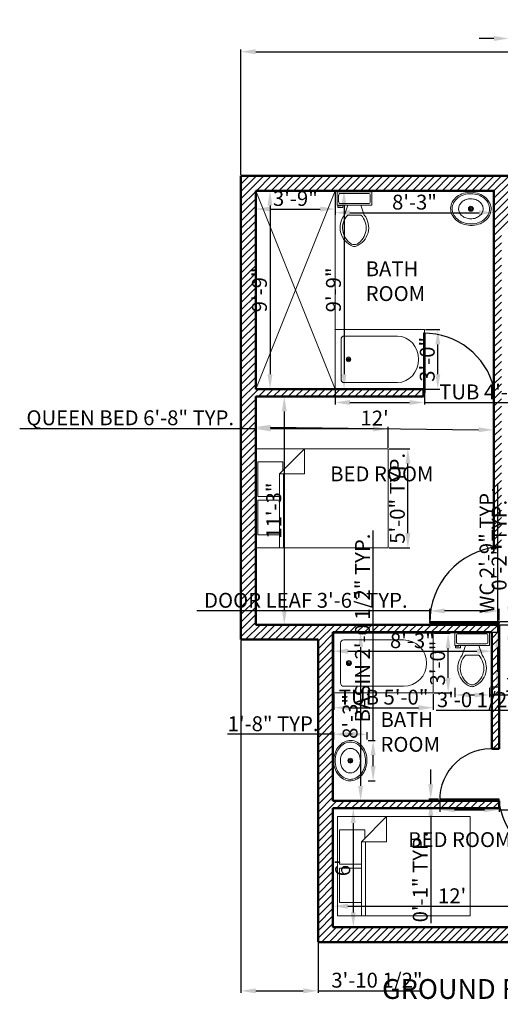
# Model space of a CAD drawing. Units: inches. Extents: x 5928 to 6612, y 5674 to 6320.
# Tile 1 of 5: x 5928 to 6219, y 5674 to 6269. Entities that reach past the tile are written whole.
import ezdxf

# ---------------------------------------------------------------- set-up
doc = ezdxf.new("R2010")
doc.units = ezdxf.units.IN
for name, color, linetype, lineweight in [('A-ANNO-DIMS', 2, 'Continuous', 18), ('A-ANNO-TEXT', 7, 'Continuous', 25), ('A-AREA-IDEN', 7, 'Continuous', 25), ('A-DOOR', 3, 'Continuous', 25), ('A-FLOR-FIXT', 9, 'Continuous', 18), ('A-FLOR-OPEN', 8, 'Continuous', 18), ('A-FURN', 8, 'Continuous', 18), ('A-WALL', 7, 'Continuous', 50), ('A-WALL-PATT', 252, 'Continuous', 13)]:
    doc.layers.add(name, color=color, linetype=linetype, lineweight=lineweight)
doc.styles.get("Standard").update_dxf_attribs({"font": 'arial.ttf'})
doc.dimstyles.new('ISO-25', dxfattribs={"dimtxt": 9, "dimasz": 9, "dimexe": 1.25, "dimexo": 0.625, "dimtad": 1, "dimdec": 1, "dimrnd": 9, "dimlunit": 3, "dimtxsty": 'Standard', "dimcen": 2.5, "dimadec": 0, "dimazin": 0, "dimtfac": 1, "dimtdec": 1, "dimtmove": 0, "dimatfit": 3, "dimfxl": 1, "dimarcsym": 0})

# ---------------------------------------------------------------- blocks, each defined once
blk = doc.blocks.new('Bed - Queen')
for p, q in [((0, -80.00003), (0, 0)), ((0, 0), (59.99999, 0)), ((59.99999, 0), (59.99999, -80.00003)), ((7.99999, -1.2), (28.79998, -1.2)), ((7.99999, -14.4), (7.99999, -1.2)), ((28.79998, -1.2), (28.79998, -14.4)), ((31.19999, -1.2), (51.99999, -1.2)), ((31.19999, -14.4), (31.19999, -1.2)), ((51.99999, -1.2), (51.99999, -16.4)), ((0, -14.4), (44.8, -14.4)), ((44.8, -16.8), (0, -16.8)), ((59.99999, -29.6), (44.8, -14.4)), ((44.8, -14.4), (44.8, -29.6)), ((51.99999, -16.4), (46.79936, -16.4)), ((44.8, -29.6), (59.99999, -29.6)), ((59.99999, -80.00003), (0, -80.00003))]:
    blk.add_line(p, q)
blk = doc.blocks.new('Toilet - top')
for p, q in [((9.5, -6), (9.5, -2)), ((-10, -8.5), (-8, -8.5)), ((-10, -9.5), (-10, -8.5)), ((-7, -9.5), (-10, -9.5)), ((-8, -8.5), (-8, -8)), ((-7, -8), (-7, -9.5)), ((-4, -8), (-6, -14)), ((4, -8), (6, -14)), ((4, -14), (-4, -14))]:
    blk.add_line(p, q)
blk.add_lwpolyline([(10.5, -8), (10.5, 0), (-10.5, 0), (-10.5, -8)], close=True)
for points in [[(-9.5, -2), (-9.5, -6)], [(8.5, -1), (-8.5, -1)], [(-8.5, -7), (8.5, -7)]]:
    blk.add_lwpolyline(points)
for centre, radius, start, end in [((-8.62, -1.88), 0.884, 81.8699, 188.1301), ((8.62, -1.88), 0.884, 351.8699, 98.1301), ((-8.62, -6.12), 0.884, 171.8699, 278.1301), ((8.62, -6.12), 0.884, 261.8699, 8.1301), ((3.52, -21.58), 12.17, 141.46911, 247.97143), ((4.2, -21.82), 11.33, 136.36773, 238.94682), ((-3.52, -21.58), 12.17, 292.02843, 38.53071), ((-4.2, -21.82), 11.33, 301.05301, 43.63209), ((0, -27.88), 4, 245.73182, 294.26817), ((0, -29), 4, 254.86053, 285.13947)]:
    blk.add_arc(centre, radius, start, end)
blk = doc.blocks.new('Bath Tub - 26 x 60 in.')
for p, q in [((9, -17), (9, -19)), ((8, -18), (10, -18))]:
    blk.add_line(p, q)
blk.add_lwpolyline([(0, -36), (0, 0), (60, 0), (60, -36)], close=True)
for points in [[(6, -4), (42, -4)], [(4, -30), (4, -6)], [(42, -32), (6, -32)]]:
    blk.add_lwpolyline(points)
for radius in [1.5, 1]:
    blk.add_circle((9, -18), radius)
for centre, radius, start, end in [((5.75, -5.75), 1.77, 81.8699, 188.1301), ((42, -18), 14, 270, 90), ((5.75, -30.25), 1.77, 171.8699, 278.1301)]:
    blk.add_arc(centre, radius, start, end)
blk = doc.blocks.new('Sink - Oval top')
for p, q in [((-1, 0), (1, 0)), ((0, 1), (0, -1))]:
    blk.add_line(p, q)
for points in [[(-12.23, 0.39, 0.117634), (-11.46, -3.36, 0.104469), (-8.88, -6.8, 0.090016), (-5.08, -9.07, 0.08192), (-0.32, -10.02, 0.08192), (4.49, -9.38, 0.090016), (8.42, -7.36, 0.104469), (11.22, -4.09, 0.117634), (12.23, -0.39, 0.117634), (11.46, 3.36, 0.104469), (8.88, 6.8, 0.090016), (5.08, 9.07, 0.08192), (0.32, 10.02, 0.08192), (-4.49, 9.38, 0.090016), (-8.42, 7.36, 0.104469), (-11.22, 4.09, 0.117634)], [(-11.29, 0.16, 0.118622), (-10.52, -3.25, 0.104678), (-8.07, -6.36, 0.089562), (-4.54, -8.37, 0.081185), (-0.13, -9.15, 0.081185), (4.3, -8.49, 0.089562), (7.89, -6.58, 0.104678), (10.42, -3.55, 0.118622), (11.29, -0.16, 0.118622), (10.52, 3.25, 0.104678), (8.07, 6.36, 0.089562), (4.54, 8.37, 0.081185), (0.13, 9.15, 0.081185), (-4.3, 8.49, 0.089562), (-7.89, 6.58, 0.104678), (-10.42, 3.55, 0.118622)], [(-7.42, 0.08, 0.118283), (-6.91, -2.17, 0.104607), (-5.29, -4.21, 0.089718), (-2.97, -5.53, 0.081436), (-0.07, -6.04, 0.081436), (2.84, -5.59, 0.089718), (5.2, -4.33, 0.104607), (6.86, -2.32, 0.118283), (7.42, -0.08, 0.118283), (6.91, 2.17, 0.104607), (5.29, 4.21, 0.089718), (2.97, 5.53, 0.081436), (0.07, 6.04, 0.081436), (-2.84, 5.59, 0.089718), (-5.2, 4.33, 0.104607), (-6.86, 2.32, 0.118283)]]:
    blk.add_lwpolyline(points, format="xyb", close=True)
for radius in [1.5, 1]:
    blk.add_circle((0, 0), radius)
blk = doc.blocks.new('*D11')
at = {"layer": 'A-ANNO-DIMS', "color": 0, "lineweight": -2, "transparency": 16777216}
for p, q in [((6071.65, 6165.76), (6080.95, 6165.76)), ((6079.7, 6156.76), (6079.7, 6054.76)), ((6071.65, 6045.76), (6080.95, 6045.76))]:
    blk.add_line(p, q, dxfattribs=at)
at = {"layer": 'A-ANNO-DIMS', "color": 0, "transparency": 16777216}
for points in [[(6078.2, 6156.76), (6081.2, 6156.76), (6079.7, 6165.76)], [(6078.2, 6054.76), (6081.2, 6054.76), (6079.7, 6045.76)]]:
    blk.add_solid(points, dxfattribs=at)
at = {"layer": 'Defpoints', "color": 0, "transparency": 16777216}
for p in [(6071.03, 6165.76), (6071.03, 6045.76), (6079.7, 6045.76)]:
    blk.add_point(p, dxfattribs=at)
at = {"layer": 'A-ANNO-DIMS', "color": 0, "transparency": 16777216, "insert": (6074.47, 6105.76), "char_height": 9, "attachment_point": 5, "rotation": 90}
blk.add_mtext('9\'-9"', dxfattribs=at)
blk = doc.blocks.new('*D12')
at = {"layer": 'A-ANNO-DIMS', "color": 0, "lineweight": -2, "transparency": 16777216}
for p, q in [((6071.03, 6165.14), (6071.03, 6153.42)), ((6119.03, 6165.14), (6119.03, 6153.42)), ((6080.03, 6154.67), (6110.03, 6154.67))]:
    blk.add_line(p, q, dxfattribs=at)
at = {"layer": 'A-ANNO-DIMS', "color": 0, "transparency": 16777216}
for points in [[(6080.03, 6156.17), (6080.03, 6153.17), (6071.03, 6154.67)], [(6110.03, 6156.17), (6110.03, 6153.17), (6119.03, 6154.67)]]:
    blk.add_solid(points, dxfattribs=at)
at = {"layer": 'Defpoints', "color": 0, "transparency": 16777216}
for p in [(6071.03, 6165.76), (6119.03, 6165.76), (6119.03, 6154.67)]:
    blk.add_point(p, dxfattribs=at)
at = {"layer": 'A-ANNO-DIMS', "color": 0, "transparency": 16777216, "insert": (6095.03, 6159.89), "char_height": 9, "attachment_point": 5}
blk.add_mtext('3\'-9"', dxfattribs=at)
blk = doc.blocks.new('*D13')
at = {"layer": 'A-ANNO-DIMS', "color": 0, "lineweight": -2, "transparency": 16777216}
for p, q in [((6119.03, 6165.14), (6119.03, 6151.2)), ((6215.03, 6165.14), (6215.03, 6151.2)), ((6128.03, 6152.45), (6206.03, 6152.45))]:
    blk.add_line(p, q, dxfattribs=at)
at = {"layer": 'A-ANNO-DIMS', "color": 0, "transparency": 16777216}
for points in [[(6128.03, 6153.95), (6128.03, 6150.95), (6119.03, 6152.45)], [(6206.03, 6153.95), (6206.03, 6150.95), (6215.03, 6152.45)]]:
    blk.add_solid(points, dxfattribs=at)
at = {"layer": 'Defpoints', "color": 0, "transparency": 16777216}
for p in [(6119.03, 6165.76), (6215.03, 6165.76), (6215.03, 6152.45)]:
    blk.add_point(p, dxfattribs=at)
at = {"layer": 'A-ANNO-DIMS', "color": 0, "transparency": 16777216, "insert": (6167.03, 6157.67), "char_height": 9, "attachment_point": 5}
blk.add_mtext('8\'-3"', dxfattribs=at)
blk = doc.blocks.new('*D14')
at = {"layer": 'A-ANNO-DIMS', "color": 0, "lineweight": -2, "transparency": 16777216}
for p, q in [((6119.65, 6165.76), (6125.68, 6165.76)), ((6124.43, 6156.76), (6124.43, 6054.76)), ((6119.65, 6045.76), (6125.68, 6045.76))]:
    blk.add_line(p, q, dxfattribs=at)
at = {"layer": 'A-ANNO-DIMS', "color": 0, "transparency": 16777216}
for points in [[(6122.93, 6156.76), (6125.93, 6156.76), (6124.43, 6165.76)], [(6122.93, 6054.76), (6125.93, 6054.76), (6124.43, 6045.76)]]:
    blk.add_solid(points, dxfattribs=at)
at = {"layer": 'Defpoints', "color": 0, "transparency": 16777216}
for p in [(6119.03, 6165.76), (6119.03, 6045.76), (6124.43, 6045.76)]:
    blk.add_point(p, dxfattribs=at)
at = {"layer": 'A-ANNO-DIMS', "color": 0, "transparency": 16777216, "insert": (6119.21, 6105.76), "char_height": 9, "attachment_point": 5, "rotation": 90}
blk.add_mtext('9\'-9"', dxfattribs=at)
blk = doc.blocks.new('*D15')
at = {"layer": 'A-ANNO-DIMS', "color": 0, "lineweight": -2, "transparency": 16777216}
for p, q in [((6071.65, 6041.26), (6089.58, 6041.26)), ((6088.33, 6032.26), (6088.33, 5912.26)), ((6071.65, 5903.26), (6089.58, 5903.26))]:
    blk.add_line(p, q, dxfattribs=at)
at = {"layer": 'A-ANNO-DIMS', "color": 0, "transparency": 16777216}
for points in [[(6086.83, 6032.26), (6089.83, 6032.26), (6088.33, 6041.26)], [(6086.83, 5912.26), (6089.83, 5912.26), (6088.33, 5903.26)]]:
    blk.add_solid(points, dxfattribs=at)
at = {"layer": 'Defpoints', "color": 0, "transparency": 16777216}
for p in [(6071.03, 6041.26), (6071.03, 5903.26), (6088.33, 5903.26)]:
    blk.add_point(p, dxfattribs=at)
at = {"layer": 'A-ANNO-DIMS', "color": 0, "transparency": 16777216, "insert": (6083.11, 5972.26), "char_height": 9, "attachment_point": 5, "rotation": 90}
blk.add_mtext('11\'-3"', dxfattribs=at)
blk = doc.blocks.new('*D16')
at = {"layer": 'A-ANNO-DIMS', "color": 0, "lineweight": -2, "transparency": 16777216}
for p, q in [((6071.02, 6040.64), (6070.8, 6021.52)), ((6215.02, 6038.94), (6214.8, 6019.82)), ((6079.81, 6022.66), (6205.81, 6021.18))]:
    blk.add_line(p, q, dxfattribs=at)
at = {"layer": 'A-ANNO-DIMS', "color": 0, "transparency": 16777216}
for points in [[(6079.83, 6024.16), (6079.79, 6021.16), (6070.81, 6022.77)], [(6205.83, 6022.68), (6205.79, 6019.68), (6214.81, 6021.07)]]:
    blk.add_solid(points, dxfattribs=at)
at = {"layer": 'Defpoints', "color": 0, "transparency": 16777216}
for p in [(6071.03, 6041.26), (6215.03, 6039.57), (6214.81, 6021.07)]:
    blk.add_point(p, dxfattribs=at)
at = {"layer": 'A-ANNO-DIMS', "color": 0, "transparency": 16777216, "insert": (6142.87, 6027.06), "char_height": 9, "attachment_point": 5, "rotation": 359.32572}
blk.add_mtext("12'", dxfattribs=at)
blk = doc.blocks.new('*D17')
at = {"layer": 'A-ANNO-DIMS', "color": 0, "lineweight": -2, "transparency": 16777216}
for p, q in [((6118.38, 5898.76), (6135.72, 5898.76)), ((6134.47, 5889.76), (6134.47, 5805.76)), ((6118.38, 5796.76), (6135.72, 5796.76))]:
    blk.add_line(p, q, dxfattribs=at)
at = {"layer": 'A-ANNO-DIMS', "color": 0, "transparency": 16777216}
for points in [[(6132.97, 5889.76), (6135.97, 5889.76), (6134.47, 5898.76)], [(6132.97, 5805.76), (6135.97, 5805.76), (6134.47, 5796.76)]]:
    blk.add_solid(points, dxfattribs=at)
at = {"layer": 'Defpoints', "color": 0, "transparency": 16777216}
for p in [(6117.76, 5898.76), (6117.76, 5796.76), (6134.47, 5796.76)]:
    blk.add_point(p, dxfattribs=at)
at = {"layer": 'A-ANNO-DIMS', "color": 0, "transparency": 16777216, "insert": (6129.25, 5847.76), "char_height": 9, "attachment_point": 5, "rotation": 90}
blk.add_mtext('8\'-3"', dxfattribs=at)
blk = doc.blocks.new('*D18')
at = {"layer": 'A-ANNO-DIMS', "color": 0, "lineweight": -2, "transparency": 16777216}
for p, q in [((6117.76, 5898.14), (6117.76, 5885.97)), ((6213.76, 5898.14), (6213.76, 5885.97)), ((6126.76, 5887.22), (6204.76, 5887.22))]:
    blk.add_line(p, q, dxfattribs=at)
at = {"layer": 'A-ANNO-DIMS', "color": 0, "transparency": 16777216}
for points in [[(6126.76, 5888.72), (6126.76, 5885.72), (6117.76, 5887.22)], [(6204.76, 5888.72), (6204.76, 5885.72), (6213.76, 5887.22)]]:
    blk.add_solid(points, dxfattribs=at)
at = {"layer": 'Defpoints', "color": 0, "transparency": 16777216}
for p in [(6117.76, 5898.76), (6213.76, 5898.76), (6213.76, 5887.22)]:
    blk.add_point(p, dxfattribs=at)
at = {"layer": 'A-ANNO-DIMS', "color": 0, "transparency": 16777216, "insert": (6165.76, 5892.44), "char_height": 9, "attachment_point": 5}
blk.add_mtext('8\'-3"', dxfattribs=at)
blk = doc.blocks.new('*D19')
at = {"layer": 'A-ANNO-DIMS', "color": 0, "lineweight": -2, "transparency": 16777216}
for p, q in [((6118.38, 5792.26), (6131.29, 5792.26)), ((6130.04, 5783.26), (6130.04, 5729.26)), ((6118.38, 5720.26), (6131.29, 5720.26))]:
    blk.add_line(p, q, dxfattribs=at)
at = {"layer": 'A-ANNO-DIMS', "color": 0, "transparency": 16777216}
for points in [[(6128.54, 5783.26), (6131.54, 5783.26), (6130.04, 5792.26)], [(6128.54, 5729.26), (6131.54, 5729.26), (6130.04, 5720.26)]]:
    blk.add_solid(points, dxfattribs=at)
at = {"layer": 'Defpoints', "color": 0, "transparency": 16777216}
for p in [(6117.76, 5792.26), (6117.76, 5720.26), (6130.04, 5720.26)]:
    blk.add_point(p, dxfattribs=at)
at = {"layer": 'A-ANNO-DIMS', "color": 0, "transparency": 16777216, "insert": (6124.82, 5756.26), "char_height": 9, "attachment_point": 5, "rotation": 90}
blk.add_mtext("6'", dxfattribs=at)
blk = doc.blocks.new('*D20')
at = {"layer": 'A-ANNO-DIMS', "color": 0, "lineweight": -2, "transparency": 16777216}
for p, q in [((6117.76, 5720.89), (6117.76, 5734.25)), ((6126.76, 5733), (6252.76, 5733)), ((6261.76, 5720.89), (6261.76, 5734.25))]:
    blk.add_line(p, q, dxfattribs=at)
at = {"layer": 'A-ANNO-DIMS', "color": 0, "transparency": 16777216}
for points in [[(6126.76, 5734.5), (6126.76, 5731.5), (6117.76, 5733)], [(6252.76, 5734.5), (6252.76, 5731.5), (6261.76, 5733)]]:
    blk.add_solid(points, dxfattribs=at)
at = {"layer": 'Defpoints', "color": 0, "transparency": 16777216}
for p in [(6261.76, 5733), (6117.76, 5720.26), (6261.76, 5720.26)]:
    blk.add_point(p, dxfattribs=at)
at = {"layer": 'A-ANNO-DIMS', "color": 0, "transparency": 16777216, "insert": (6189.76, 5738.14), "char_height": 9, "attachment_point": 5}
blk.add_mtext("12'", dxfattribs=at)
blk = doc.blocks.new('*D36')
at = {"layer": 'A-ANNO-DIMS', "color": 0, "lineweight": -2, "transparency": 16777216}
for p, q in [((6062.03, 6175.39), (6062.03, 6251.06)), ((6071.03, 6249.81), (6539.03, 6249.81)), ((6548.03, 6176.51), (6548.03, 6251.06))]:
    blk.add_line(p, q, dxfattribs=at)
at = {"layer": 'A-ANNO-DIMS', "color": 0, "transparency": 16777216}
for points in [[(6071.03, 6251.31), (6071.03, 6248.31), (6062.03, 6249.81)], [(6539.03, 6251.31), (6539.03, 6248.31), (6548.03, 6249.81)]]:
    blk.add_solid(points, dxfattribs=at)
at = {"layer": 'Defpoints', "color": 0, "transparency": 16777216}
for p in [(6548.03, 6249.81), (6548.03, 6175.89), (6062.03, 6174.76)]:
    blk.add_point(p, dxfattribs=at)
at = {"layer": 'A-ANNO-DIMS', "color": 0, "transparency": 16777216, "insert": (6305.03, 6255.03), "char_height": 9, "attachment_point": 5}
blk.add_mtext('40\'-6"', dxfattribs=at)
blk = doc.blocks.new('DOOR-LEAF-42IN')
for p, q in [((0, 0), (0, 42)), ((0, 42), (1, 42)), ((1, 42), (1, 0)), ((-1, 0), (0, 0)), ((1, 0), (0, 0))]:
    blk.add_line(p, q)
blk = doc.blocks.new('DOOR-LEAF-FLUSH-36IN')
for p, q in [((0, 0), (-1, 0)), ((-1, 0), (-1, -36)), ((-1, -36), (0, -36))]:
    blk.add_line(p, q)
blk = doc.blocks.new('*D42')
at = {"layer": 'A-ANNO-DIMS', "color": 0, "lineweight": -2, "transparency": 16777216}
for p, q in [((6142.01, 5833.29), (6142.01, 5960.2)), ((6138.96, 5833.29), (6143.26, 5833.29)), ((6142.01, 5817.74), (6142.01, 5824.29)), ((6138.96, 5808.74), (6143.26, 5808.74))]:
    blk.add_line(p, q, dxfattribs=at)
at = {"layer": 'A-ANNO-DIMS', "color": 0, "transparency": 16777216}
for points in [[(6140.51, 5824.29), (6143.51, 5824.29), (6142.01, 5833.29)], [(6140.51, 5817.74), (6143.51, 5817.74), (6142.01, 5808.74)]]:
    blk.add_solid(points, dxfattribs=at)
at = {"layer": 'Defpoints', "color": 0, "transparency": 16777216}
for p in [(6138.33, 5833.29), (6142.01, 5833.29), (6138.33, 5808.74)]:
    blk.add_point(p, dxfattribs=at)
at = {"layer": 'A-ANNO-DIMS', "color": 0, "transparency": 16777216, "insert": (6136.74, 5901.25), "char_height": 9, "attachment_point": 5, "rotation": 90}
blk.add_mtext('BASIN 2\'-0 1/2" TYP.', dxfattribs=at)
blk = doc.blocks.new('*D43')
at = {"layer": 'A-ANNO-DIMS', "color": 0, "lineweight": -2, "transparency": 16777216}
for p, q in [((6118.19, 5836.98), (6053.93, 5836.98)), ((6118.19, 5833.92), (6118.19, 5838.23)), ((6129.33, 5836.98), (6127.19, 5836.98)), ((6138.33, 5833.92), (6138.33, 5838.23))]:
    blk.add_line(p, q, dxfattribs=at)
at = {"layer": 'A-ANNO-DIMS', "color": 0, "transparency": 16777216}
for points in [[(6127.19, 5838.48), (6127.19, 5835.48), (6118.19, 5836.98)], [(6129.33, 5838.48), (6129.33, 5835.48), (6138.33, 5836.98)]]:
    blk.add_solid(points, dxfattribs=at)
at = {"layer": 'Defpoints', "color": 0, "transparency": 16777216}
for p in [(6118.19, 5836.98), (6118.19, 5833.29), (6138.33, 5833.29)]:
    blk.add_point(p, dxfattribs=at)
at = {"layer": 'A-ANNO-DIMS', "color": 0, "transparency": 16777216, "insert": (6081.56, 5842.2), "char_height": 9, "attachment_point": 5}
blk.add_mtext('1\'-8" TYP.', dxfattribs=at)
blk = doc.blocks.new('*D44')
at = {"layer": 'A-ANNO-DIMS', "color": 0, "lineweight": -2, "transparency": 16777216}
for p, q in [((6176.26, 5911.56), (6035.45, 5911.56)), ((6176.26, 5905.89), (6176.26, 5912.81)), ((6209.26, 5911.56), (6185.26, 5911.56)), ((6218.26, 5905.89), (6218.26, 5912.81))]:
    blk.add_line(p, q, dxfattribs=at)
at = {"layer": 'A-ANNO-DIMS', "color": 0, "transparency": 16777216}
for points in [[(6185.26, 5913.06), (6185.26, 5910.06), (6176.26, 5911.56)], [(6209.26, 5913.06), (6209.26, 5910.06), (6218.26, 5911.56)]]:
    blk.add_solid(points, dxfattribs=at)
at = {"layer": 'Defpoints', "color": 0, "transparency": 16777216}
for p in [(6176.26, 5911.56), (6176.26, 5905.26), (6218.26, 5905.26)]:
    blk.add_point(p, dxfattribs=at)
at = {"layer": 'A-ANNO-DIMS', "color": 0, "transparency": 16777216, "insert": (6101.35, 5916.85), "char_height": 9, "attachment_point": 5}
blk.add_mtext('DOOR LEAF 3\'-6" TYP.', dxfattribs=at)
blk = doc.blocks.new('*D45')
at = {"layer": 'A-ANNO-DIMS', "color": 0, "lineweight": -2, "transparency": 16777216}
for p, q in [((6224.56, 5914.26), (6224.56, 5979.37)), ((6218.88, 5905.26), (6225.81, 5905.26)), ((6218.88, 5903.26), (6225.81, 5903.26)), ((6224.56, 5903.26), (6224.56, 5905.26)), ((6224.56, 5894.26), (6224.56, 5885.26))]:
    blk.add_line(p, q, dxfattribs=at)
at = {"layer": 'A-ANNO-DIMS', "color": 0, "transparency": 16777216}
for points in [[(6223.06, 5914.26), (6226.06, 5914.26), (6224.56, 5905.26)], [(6223.06, 5894.26), (6226.06, 5894.26), (6224.56, 5903.26)]]:
    blk.add_solid(points, dxfattribs=at)
at = {"layer": 'Defpoints', "color": 0, "transparency": 16777216}
for p in [(6218.26, 5905.26), (6218.26, 5903.26), (6224.56, 5905.26)]:
    blk.add_point(p, dxfattribs=at)
at = {"layer": 'A-ANNO-DIMS', "color": 0, "transparency": 16777216, "insert": (6219.34, 5951.32), "char_height": 9, "attachment_point": 5, "rotation": 90}
blk.add_mtext('0\'-2" TYP.', dxfattribs=at)
blk = doc.blocks.new('*D46')
at = {"layer": 'A-ANNO-DIMS', "color": 0, "lineweight": -2, "transparency": 16777216}
for p, q in [((6071.03, 6021.69), (5928.39, 6021.69)), ((6071.03, 6010.32), (6071.03, 6022.94)), ((6142.03, 6021.69), (6080.03, 6021.69)), ((6151.03, 6010.32), (6151.03, 6022.94))]:
    blk.add_line(p, q, dxfattribs=at)
at = {"layer": 'A-ANNO-DIMS', "color": 0, "transparency": 16777216}
for points in [[(6080.03, 6023.19), (6080.03, 6020.19), (6071.03, 6021.69)], [(6142.03, 6023.19), (6142.03, 6020.19), (6151.03, 6021.69)]]:
    blk.add_solid(points, dxfattribs=at)
at = {"layer": 'Defpoints', "color": 0, "transparency": 16777216}
for p in [(6071.03, 6021.69), (6071.03, 6009.69), (6151.03, 6009.69)]:
    blk.add_point(p, dxfattribs=at)
at = {"layer": 'A-ANNO-DIMS', "color": 0, "transparency": 16777216, "insert": (5995.21, 6027.25), "char_height": 9, "attachment_point": 5}
blk.add_mtext('QUEEN BED 6\'-8" TYP.', dxfattribs=at)
blk = doc.blocks.new('*D47')
at = {"layer": 'A-ANNO-DIMS', "color": 0, "lineweight": -2, "transparency": 16777216}
for p, q in [((6151.65, 6009.69), (6164.28, 6009.69)), ((6163.03, 5958.69), (6163.03, 6000.69)), ((6151.65, 5949.69), (6164.28, 5949.69))]:
    blk.add_line(p, q, dxfattribs=at)
at = {"layer": 'A-ANNO-DIMS', "color": 0, "transparency": 16777216}
for points in [[(6161.53, 6000.69), (6164.53, 6000.69), (6163.03, 6009.69)], [(6161.53, 5958.69), (6164.53, 5958.69), (6163.03, 5949.69)]]:
    blk.add_solid(points, dxfattribs=at)
at = {"layer": 'Defpoints', "color": 0, "transparency": 16777216}
for p in [(6151.03, 6009.69), (6163.03, 6009.69), (6151.03, 5949.69)]:
    blk.add_point(p, dxfattribs=at)
at = {"layer": 'A-ANNO-DIMS', "color": 0, "transparency": 16777216, "insert": (6157.81, 5979.69), "char_height": 9, "attachment_point": 5, "rotation": 90}
blk.add_mtext('5\'-0" TYP.', dxfattribs=at)
blk = doc.blocks.new('*D48')
at = {"layer": 'A-ANNO-DIMS', "color": 0, "lineweight": -2, "transparency": 16777216}
for p, q in [((6217.31, 5898.76), (6217.31, 5988.68)), ((6212.98, 5898.76), (6218.56, 5898.76)), ((6217.31, 5874.72), (6217.31, 5889.76)), ((6212.98, 5865.72), (6218.56, 5865.72))]:
    blk.add_line(p, q, dxfattribs=at)
at = {"layer": 'A-ANNO-DIMS', "color": 0, "transparency": 16777216}
for points in [[(6215.81, 5889.76), (6218.81, 5889.76), (6217.31, 5898.76)], [(6215.81, 5874.72), (6218.81, 5874.72), (6217.31, 5865.72)]]:
    blk.add_solid(points, dxfattribs=at)
at = {"layer": 'Defpoints', "color": 0, "transparency": 16777216}
for p in [(6212.35, 5898.76), (6217.31, 5898.76), (6212.35, 5865.72)]:
    blk.add_point(p, dxfattribs=at)
at = {"layer": 'A-ANNO-DIMS', "color": 0, "transparency": 16777216, "insert": (6212.03, 5948.22), "char_height": 9, "attachment_point": 5, "rotation": 90}
blk.add_mtext('WC 2\'-9" TYP.', dxfattribs=at)
blk = doc.blocks.new('*D49')
at = {"layer": 'A-ANNO-DIMS', "color": 0, "lineweight": -2, "transparency": 16777216}
for p, q in [((6191.35, 5865.09), (6191.35, 5859.51)), ((6200.35, 5860.76), (6203.35, 5860.76)), ((6212.35, 5865.09), (6212.35, 5859.51)), ((6212.35, 5860.76), (6276.61, 5860.76))]:
    blk.add_line(p, q, dxfattribs=at)
at = {"layer": 'A-ANNO-DIMS', "color": 0, "transparency": 16777216}
for points in [[(6200.35, 5862.26), (6200.35, 5859.26), (6191.35, 5860.76)], [(6203.35, 5862.26), (6203.35, 5859.26), (6212.35, 5860.76)]]:
    blk.add_solid(points, dxfattribs=at)
at = {"layer": 'Defpoints', "color": 0, "transparency": 16777216}
for p in [(6191.35, 5865.72), (6212.35, 5865.72), (6212.35, 5860.76)]:
    blk.add_point(p, dxfattribs=at)
at = {"layer": 'A-ANNO-DIMS', "color": 0, "transparency": 16777216, "insert": (6248.98, 5865.98), "char_height": 9, "attachment_point": 5}
blk.add_mtext('1\'-9" TYP.', dxfattribs=at)
blk = doc.blocks.new('*D50')
at = {"layer": 'A-ANNO-DIMS', "color": 0, "lineweight": -2, "transparency": 16777216}
for p, q in [((6119.03, 6045.14), (6119.03, 6036.41)), ((6173.03, 6045.14), (6173.03, 6036.41)), ((6128.03, 6037.66), (6164.03, 6037.66)), ((6173.03, 6037.66), (6236.07, 6037.66))]:
    blk.add_line(p, q, dxfattribs=at)
at = {"layer": 'A-ANNO-DIMS', "color": 0, "transparency": 16777216}
for points in [[(6128.03, 6039.16), (6128.03, 6036.16), (6119.03, 6037.66)], [(6164.03, 6039.16), (6164.03, 6036.16), (6173.03, 6037.66)]]:
    blk.add_solid(points, dxfattribs=at)
at = {"layer": 'Defpoints', "color": 0, "transparency": 16777216}
for p in [(6119.03, 6045.76), (6173.03, 6045.76), (6173.03, 6037.66)]:
    blk.add_point(p, dxfattribs=at)
at = {"layer": 'A-ANNO-DIMS', "color": 0, "transparency": 16777216, "insert": (6209.05, 6042.88), "char_height": 9, "attachment_point": 5}
blk.add_mtext('TUB 4\'-6"', dxfattribs=at)
blk = doc.blocks.new('*D51')
at = {"layer": 'A-ANNO-DIMS', "color": 0, "lineweight": -2, "transparency": 16777216}
for p, q in [((6173.65, 6081.76), (6182.38, 6081.76)), ((6181.13, 6054.76), (6181.13, 6072.76)), ((6173.65, 6045.76), (6182.38, 6045.76))]:
    blk.add_line(p, q, dxfattribs=at)
at = {"layer": 'A-ANNO-DIMS', "color": 0, "transparency": 16777216}
for points in [[(6179.63, 6072.76), (6182.63, 6072.76), (6181.13, 6081.76)], [(6179.63, 6054.76), (6182.63, 6054.76), (6181.13, 6045.76)]]:
    blk.add_solid(points, dxfattribs=at)
at = {"layer": 'Defpoints', "color": 0, "transparency": 16777216}
for p in [(6173.03, 6081.76), (6181.13, 6081.76), (6173.03, 6045.76)]:
    blk.add_point(p, dxfattribs=at)
at = {"layer": 'A-ANNO-DIMS', "color": 0, "transparency": 16777216, "insert": (6175.9, 6063.76), "char_height": 9, "attachment_point": 5, "rotation": 90}
blk.add_mtext('3\'-0"', dxfattribs=at)
blk = doc.blocks.new('*D52')
at = {"layer": 'A-ANNO-DIMS', "color": 0, "lineweight": -2, "transparency": 16777216}
for p, q in [((6118.36, 5861.43), (6118.36, 5851.8)), ((6178.36, 5861.43), (6178.36, 5851.8)), ((6127.36, 5853.05), (6169.36, 5853.05))]:
    blk.add_line(p, q, dxfattribs=at)
at = {"layer": 'A-ANNO-DIMS', "color": 0, "transparency": 16777216}
for points in [[(6127.36, 5854.55), (6127.36, 5851.55), (6118.36, 5853.05)], [(6169.36, 5854.55), (6169.36, 5851.55), (6178.36, 5853.05)]]:
    blk.add_solid(points, dxfattribs=at)
at = {"layer": 'Defpoints', "color": 0, "transparency": 16777216}
for p in [(6118.36, 5862.05), (6178.36, 5862.05), (6178.36, 5853.05)]:
    blk.add_point(p, dxfattribs=at)
at = {"layer": 'A-ANNO-DIMS', "color": 0, "transparency": 16777216, "insert": (6148.36, 5858.27), "char_height": 9, "attachment_point": 5}
blk.add_mtext('TUB 5\'-0"', dxfattribs=at)
blk = doc.blocks.new('*D53')
at = {"layer": 'A-ANNO-DIMS', "color": 0, "lineweight": -2, "transparency": 16777216}
for p, q in [((6178.99, 5898.05), (6188.61, 5898.05)), ((6187.36, 5871.05), (6187.36, 5889.05)), ((6178.99, 5862.05), (6188.61, 5862.05))]:
    blk.add_line(p, q, dxfattribs=at)
at = {"layer": 'A-ANNO-DIMS', "color": 0, "transparency": 16777216}
for points in [[(6185.86, 5889.05), (6188.86, 5889.05), (6187.36, 5898.05)], [(6185.86, 5871.05), (6188.86, 5871.05), (6187.36, 5862.05)]]:
    blk.add_solid(points, dxfattribs=at)
at = {"layer": 'Defpoints', "color": 0, "transparency": 16777216}
for p in [(6178.36, 5898.05), (6187.36, 5898.05), (6178.36, 5862.05)]:
    blk.add_point(p, dxfattribs=at)
at = {"layer": 'A-ANNO-DIMS', "color": 0, "transparency": 16777216, "insert": (6182.14, 5880.05), "char_height": 9, "attachment_point": 5, "rotation": 90}
blk.add_mtext('3\'-0"', dxfattribs=at)
blk = doc.blocks.new('*D55')
at = {"layer": 'A-ANNO-DIMS', "color": 0, "lineweight": -2, "transparency": 16777216}
for p, q in [((6266.17, 5851.43), (6180.09, 5851.43)), ((6266.17, 5839.46), (6266.17, 5852.68)), ((6293.83, 5851.43), (6275.17, 5851.43)), ((6302.83, 5839.46), (6302.83, 5852.68))]:
    blk.add_line(p, q, dxfattribs=at)
at = {"layer": 'A-ANNO-DIMS', "color": 0, "transparency": 16777216}
for points in [[(6275.17, 5852.93), (6275.17, 5849.93), (6266.17, 5851.43)], [(6293.83, 5852.93), (6293.83, 5849.93), (6302.83, 5851.43)]]:
    blk.add_solid(points, dxfattribs=at)
at = {"layer": 'Defpoints', "color": 0, "transparency": 16777216}
for p in [(6266.17, 5851.43), (6266.17, 5838.83), (6302.83, 5838.83)]:
    blk.add_point(p, dxfattribs=at)
at = {"layer": 'A-ANNO-DIMS', "color": 0, "transparency": 16777216, "insert": (6218.63, 5856.72), "char_height": 9, "attachment_point": 5, "rotation": 359.99997}
blk.add_mtext('3\'-0 1/2" TYP.', dxfattribs=at)
blk = doc.blocks.new('*D60')
at = {"layer": 'A-ANNO-DIMS', "color": 0, "lineweight": -2, "transparency": 16777216}
for p, q in [((6182.26, 5796.14), (6182.26, 5790.11)), ((6218.26, 5796.14), (6218.26, 5790.11)), ((6191.26, 5791.36), (6209.26, 5791.36)), ((6218.26, 5791.36), (6362.51, 5791.36))]:
    blk.add_line(p, q, dxfattribs=at)
at = {"layer": 'A-ANNO-DIMS', "color": 0, "transparency": 16777216}
for points in [[(6191.26, 5792.86), (6191.26, 5789.86), (6182.26, 5791.36)], [(6209.26, 5792.86), (6209.26, 5789.86), (6218.26, 5791.36)]]:
    blk.add_solid(points, dxfattribs=at)
at = {"layer": 'Defpoints', "color": 0, "transparency": 16777216}
for p in [(6182.26, 5796.76), (6218.26, 5796.76), (6218.26, 5791.36)]:
    blk.add_point(p, dxfattribs=at)
at = {"layer": 'A-ANNO-DIMS', "color": 0, "transparency": 16777216, "insert": (6294.88, 5796.65), "char_height": 9, "attachment_point": 5}
blk.add_mtext('FLUSH LEAF 3\'-0" TYP.', dxfattribs=at)
blk = doc.blocks.new('*D61')
at = {"layer": 'A-ANNO-DIMS', "color": 0, "lineweight": -2, "transparency": 16777216}
for p, q in [((6176.86, 5806.76), (6176.86, 5815.76)), ((6181.63, 5797.76), (6175.61, 5797.76)), ((6181.63, 5796.76), (6175.61, 5796.76)), ((6176.86, 5797.76), (6176.86, 5796.76)), ((6176.86, 5787.76), (6176.86, 5722.65))]:
    blk.add_line(p, q, dxfattribs=at)
at = {"layer": 'A-ANNO-DIMS', "color": 0, "transparency": 16777216}
for points in [[(6175.36, 5806.76), (6178.36, 5806.76), (6176.86, 5797.76)], [(6175.36, 5787.76), (6178.36, 5787.76), (6176.86, 5796.76)]]:
    blk.add_solid(points, dxfattribs=at)
at = {"layer": 'Defpoints', "color": 0, "transparency": 16777216}
for p in [(6176.86, 5796.76), (6182.26, 5797.76), (6182.26, 5796.76)]:
    blk.add_point(p, dxfattribs=at)
at = {"layer": 'A-ANNO-DIMS', "color": 0, "transparency": 16777216, "insert": (6171.64, 5750.71), "char_height": 9, "attachment_point": 5, "rotation": 90}
blk.add_mtext('0\'-1" TYP.', dxfattribs=at)
blk = doc.blocks.new('*D72')
at = {"layer": 'A-ANNO-DIMS', "color": 0, "lineweight": -2, "transparency": 16777216}
for p, q in [((6062.03, 5893.64), (6062.03, 5680.56)), ((6108.76, 5710.64), (6108.76, 5680.56)), ((6071.03, 5681.81), (6099.76, 5681.81)), ((6108.76, 5681.81), (6170.89, 5681.81))]:
    blk.add_line(p, q, dxfattribs=at)
at = {"layer": 'A-ANNO-DIMS', "color": 0, "transparency": 16777216}
for points in [[(6071.03, 5683.31), (6071.03, 5680.31), (6062.03, 5681.81)], [(6099.76, 5683.31), (6099.76, 5680.31), (6108.76, 5681.81)]]:
    blk.add_solid(points, dxfattribs=at)
at = {"layer": 'Defpoints', "color": 0, "transparency": 16777216}
for p in [(6062.03, 5894.26), (6108.76, 5711.26), (6108.76, 5681.81)]:
    blk.add_point(p, dxfattribs=at)
at = {"layer": 'A-ANNO-DIMS', "color": 0, "transparency": 16777216, "insert": (6144.33, 5687.1), "char_height": 9, "attachment_point": 5}
blk.add_mtext('3\'-10 1/2"', dxfattribs=at)
blk = doc.blocks.new('*D73')
at = {"layer": 'A-ANNO-DIMS', "color": 0, "lineweight": -2, "transparency": 16777216}
for p, q in [((6224.03, 6175.39), (6224.03, 6259.07)), ((6239.11, 6196.83), (6239.11, 6259.07)), ((6215.03, 6257.82), (6206.03, 6257.82)), ((6224.03, 6257.82), (6239.11, 6257.82)), ((6248.11, 6257.82), (6281.43, 6257.82))]:
    blk.add_line(p, q, dxfattribs=at)
at = {"layer": 'A-ANNO-DIMS', "color": 0, "transparency": 16777216}
for points in [[(6215.03, 6259.32), (6215.03, 6256.32), (6224.03, 6257.82)], [(6248.11, 6259.32), (6248.11, 6256.32), (6239.11, 6257.82)]]:
    blk.add_solid(points, dxfattribs=at)
at = {"layer": 'Defpoints', "color": 0, "transparency": 16777216}
for p in [(6239.11, 6257.82), (6239.11, 6196.21), (6224.03, 6174.76)]:
    blk.add_point(p, dxfattribs=at)
at = {"layer": 'A-ANNO-DIMS', "color": 0, "transparency": 16777216, "insert": (6269.27, 6263.04), "char_height": 9, "attachment_point": 5}
blk.add_mtext('1\'-3"', dxfattribs=at)

msp = doc.modelspace()

# ---------------------------------------------------------------- hatches: boundary and pattern name
at = {"layer": 'A-WALL-PATT'}
h = msp.add_hatch(dxfattribs=at)
h.set_pattern_fill('ANSI31', color=256)
h.paths.add_polyline_path([(6071.03, 6165.76), (6215.03, 6165.76), (6215.03, 5969.77), (6215.03, 5950.32), (6219.53, 5950.32), (6219.53, 6142.76), (6239.11, 6142.76), (6239.11, 6151.76), (6224.03, 6151.76), (6224.03, 6174.76), (6062.03, 6174.76), (6062.03, 5969.76), (6062.03, 5894.26), (6108.76, 5894.26), (6108.76, 5711.26), (6423.76, 5711.26), (6423.76, 5750.35), (6414.76, 5750.35), (6414.76, 5720.26), (6266.26, 5720.26), (6266.26, 5862.26), (6361.1, 5862.26), (6361.1, 5866.76), (6261.76, 5866.76), (6261.76, 5720.26), (6117.76, 5720.26), (6117.76, 5792.26), (6218.26, 5792.26), (6218.26, 5796.76), (6117.76, 5796.76), (6117.76, 5898.76), (6213.76, 5898.76), (6213.76, 5828.21, -0.018207), (6216.01, 5828.09), (6218.26, 5828.09), (6218.26, 5903.26), (6117.76, 5903.26), (6071.03, 5903.26), (6071.03, 5969.77), (6071.03, 6041.26), (6117.76, 6041.26), (6172.44, 6041.26), (6172.44, 6045.76), (6117.76, 6045.76), (6071.03, 6045.76)])
h.paths.add_polyline_path([(6368.03, 6219.26), (6488.03, 6219.26), (6488.03, 6147.26), (6403.79, 6147.26), (6403.79, 6142.76), (6488.03, 6142.76), (6488.03, 5974.76), (6363.53, 5974.76), (6363.53, 5970.11), (6497.03, 5970.26), (6497.03, 6142.76), (6497.03, 6228.26), (6359.03, 6228.26), (6359.03, 6151.76), (6344.11, 6151.76), (6344.11, 6142.76), (6363.53, 6142.76), (6363.53, 6013.35), (6368.03, 6013.35), (6368.03, 6142.76)])
h.paths.add_polyline_path([(6344.11, 6196.21, 0.265753), (6295.16, 6228.26), (6288.06, 6228.26, 0.265753), (6239.11, 6196.21), (6239.11, 6142.76), (6243.61, 6142.76), (6243.61, 6196.76), (6243.45, 6196.76, -0.514089), (6339.79, 6196.74), (6339.61, 6196.76), (6339.61, 6142.76), (6344.11, 6142.76)])
h.paths.add_polyline_path([(6339.61, 6147.26), (6327.61, 6147.26), (6327.61, 6142.76), (6339.61, 6142.76)], flags=17)
h.paths.add_polyline_path([(6255.61, 6147.26), (6243.61, 6147.26), (6243.61, 6142.76), (6255.61, 6142.76)], flags=17)
h.paths.add_polyline_path([(6548.03, 5974.76), (6539.03, 5974.76), (6539.03, 5862.26), (6407.03, 5862.26), (6407.03, 5853.26), (6414.76, 5853.26), (6414.76, 5820.79), (6423.76, 5820.79), (6423.76, 5853.26), (6548.03, 5853.26)])

# ---------------------------------------------------------------- linework, layer by layer
at = {"layer": 'A-DOOR'}
for p, q in [((6173.44, 6079.51), (6172.44, 6079.51)), ((6172.44, 6079.51), (6172.44, 6045.76)), ((6173.44, 6043.51), (6173.44, 6079.51)), ((6172.44, 6043.51), (6173.44, 6043.51))]:
    msp.add_line(p, q, dxfattribs=at)
for centre, radius, start, end in [((6172.94, 6036.21), 43.31, 13.63382, 90.66151), ((6222.06, 5904.76), 45.81, 95.99605, 180.62543), ((6213.21, 5797.26), 30.95, 84.80375, 180.92563), ((6261.26, 5802.19), 43.68, 190.12275, 270.65587)]:
    msp.add_arc(centre, radius, start, end, dxfattribs=at)
at = {"layer": 'A-FLOR-OPEN'}
for p, q in [((6119.03, 6165.76), (6071.03, 6045.76)), ((6119.03, 6045.76), (6071.03, 6165.76)), ((6119.03, 6165.76), (6119.03, 6045.76))]:
    msp.add_line(p, q, dxfattribs=at)
at = {"layer": 'A-WALL'}
for p, q in [((6062.03, 6174.76), (6062.03, 5969.76)), ((6062.03, 6174.76), (6224.03, 6174.76)), ((6071.03, 6165.76), (6071.03, 6045.76)), ((6071.03, 6165.76), (6215.03, 6165.76)), ((6215.03, 6165.76), (6215.03, 5969.77)), ((6117.76, 6045.76), (6071.03, 6045.76)), ((6117.76, 6045.76), (6172.44, 6045.76)), ((6172.44, 6045.76), (6172.44, 6041.26)), ((6117.76, 6041.26), (6071.03, 6041.26)), ((6071.03, 6041.26), (6071.03, 5969.77)), ((6117.76, 6041.26), (6172.44, 6041.26)), ((6062.03, 5969.77), (6062.03, 5894.26)), ((6071.03, 5969.77), (6071.03, 5903.26)), ((6215.03, 5969.77), (6215.03, 5950.32)), ((6215.03, 5950.32), (6219.53, 5950.32)), ((6117.76, 5903.26), (6071.03, 5903.26)), ((6117.76, 5903.26), (6218.26, 5903.26)), ((6218.26, 5903.26), (6218.26, 5828.09)), ((6117.76, 5898.76), (6117.76, 5796.76)), ((6117.76, 5898.76), (6213.76, 5898.76)), ((6213.76, 5898.76), (6213.76, 5828.09)), ((6108.76, 5894.26), (6062.03, 5894.26)), ((6108.76, 5894.26), (6108.76, 5711.26)), ((6218.26, 5828.09), (6213.76, 5828.09)), ((6117.76, 5796.76), (6218.26, 5796.76)), ((6218.26, 5796.76), (6218.26, 5792.26)), ((6117.76, 5792.26), (6218.26, 5792.26)), ((6117.76, 5792.26), (6117.76, 5720.26)), ((6117.76, 5720.26), (6261.76, 5720.26)), ((6108.76, 5711.26), (6423.76, 5711.26))]:
    msp.add_line(p, q, dxfattribs=at)

# ---------------------------------------------------------------- block references
at = {"layer": 'A-DOOR'}
for name, p, rotation in [('DOOR-LEAF-42IN', (6218.26, 5904.26), 90.00000000000217), ('DOOR-LEAF-FLUSH-36IN', (6218.26, 5796.76), 270.0000000000027)]:
    msp.add_blockref(name, p, dxfattribs=dict(at, rotation=rotation))
at = {"layer": 'A-FLOR-FIXT'}
for name, p in [('Toilet - top', (6130.69, 6165.04)), ('Sink - Oval top', (6201.11, 6154.8)), ('Bath Tub - 26 x 60 in.', (6118.36, 5898.05)), ('Toilet - top', (6201.85, 5898.76))]:
    msp.add_blockref(name, p, dxfattribs=at)
at = {"layer": 'A-FLOR-FIXT', "xscale": 0.9}
msp.add_blockref('Bath Tub - 26 x 60 in.', (6119.03, 6081.76), dxfattribs=at)
at = {"layer": 'A-FLOR-FIXT', "rotation": 90}
msp.add_blockref('Sink - Oval top', (6128.26, 5821.02), dxfattribs=at)
at = {"layer": 'A-FURN', "rotation": 90}
for p in [(6071.03, 5949.69), (6120.58, 5727.23)]:
    msp.add_blockref('Bed - Queen', p, dxfattribs=at)

# ---------------------------------------------------------------- texts
at = {"layer": 'A-ANNO-TEXT', "insert": (6147.39, 5688.94), "char_height": 12, "attachment_point": 1}
msp.add_mtext_dynamic_manual_height_columns('GROUND FLOOR PLAN', width=356.796, gutter_width=12.5, heights=[0], dxfattribs=at)
at = {"layer": 'A-AREA-IDEN', "char_height": 9, "attachment_point": 1}
for s, width, heights, insert in [('BATH\\PROOM', 64.9053, [0], (6137.52, 6123.02)), ('BED ROOM', 83.8958, [0], (6116.06, 5998.98)), ('BATH\\PROOM', 64.9053, [0], (6146.46, 5850.4)), ('BED ROOM', 64.9053, [24.31], (6163.21, 5777.76))]:
    msp.add_mtext_dynamic_manual_height_columns(s, width=width, gutter_width=12.5, heights=heights, dxfattribs=dict(at, insert=insert))

# ---------------------------------------------------------------- dimensions: what is measured, and where the dimension line sits
at = {"layer": 'A-ANNO-DIMS'}
for base, p1, p2, override, picture, middle in [((6239.11, 6257.82), (6224.03, 6174.76), (6239.11, 6196.21), {"dimdec": 1, "dimlfac": 1, "dimrnd": 0, "dimzin": 1, "dimdsep": 46, "dimlunit": 4, "dimfrac": 2}, '*D73', (6269.27, 6263.04)), ((6548.03, 6249.81), (6062.03, 6174.76), (6548.03, 6175.89), {"dimclrd": 0, "dimclre": 0, "dimclrt": 0}, '*D36', (6305.03, 6255.03)), ((6119.03, 6154.67), (6071.03, 6165.76), (6119.03, 6165.76), {"dimclrd": 0, "dimclre": 0, "dimclrt": 0}, '*D12', (6095.03, 6159.89)), ((6215.03, 6152.45), (6119.03, 6165.76), (6215.03, 6165.76), {"dimclrd": 0, "dimclre": 0, "dimclrt": 0}, '*D13', (6167.03, 6157.67)), ((6213.76, 5887.22), (6117.76, 5898.76), (6213.76, 5898.76), {"dimclrd": 0, "dimclre": 0, "dimclrt": 0}, '*D18', (6165.76, 5892.44)), ((6108.76, 5681.81), (6062.03, 5894.26), (6108.76, 5711.26), {"dimdec": 1, "dimlfac": 1, "dimrnd": 0, "dimzin": 1, "dimdsep": 46, "dimlunit": 4, "dimfrac": 2}, '*D72', (6144.33, 5687.1)), ((6261.76, 5733), (6117.76, 5720.26), (6261.76, 5720.26), {"dimclrd": 0, "dimclre": 0, "dimclrt": 0}, '*D20', (6189.76, 5738.14))]:
    dim = msp.add_linear_dim(base=base, p1=p1, p2=p2, dimstyle='ISO-25', override=override, dxfattribs=at)
    dim.commit()
    dim.dimension.update_dxf_attribs({"geometry": picture, "text_midpoint": middle})
for base, p1, p2, override, picture, middle in [((6079.7, 6045.76), (6071.03, 6165.76), (6071.03, 6045.76), {"dimclrd": 0, "dimclre": 0, "dimclrt": 0}, '*D11', (6074.47, 6105.76)), ((6124.43, 6045.76), (6119.03, 6165.76), (6119.03, 6045.76), {"dimclrd": 0, "dimclre": 0, "dimclrt": 0}, '*D14', (6119.21, 6105.76)), ((6181.13, 6081.76), (6173.03, 6045.76), (6173.03, 6081.76), {"dimdec": 1, "dimlfac": 1, "dimrnd": 0, "dimzin": 1, "dimdsep": 46, "dimlunit": 4, "dimfrac": 2}, '*D51', (6175.9, 6063.76)), ((6088.33, 5903.26), (6071.03, 6041.26), (6071.03, 5903.26), {"dimclrd": 0, "dimclre": 0, "dimclrt": 0}, '*D15', (6083.11, 5972.26)), ((6134.47, 5796.76), (6117.76, 5898.76), (6117.76, 5796.76), {"dimclrd": 0, "dimclre": 0, "dimclrt": 0}, '*D17', (6129.25, 5847.76)), ((6187.36, 5898.05), (6178.36, 5862.05), (6178.36, 5898.05), {"dimdec": 1, "dimlfac": 1, "dimrnd": 0, "dimzin": 1, "dimdsep": 46, "dimlunit": 4, "dimfrac": 2}, '*D53', (6182.14, 5880.05)), ((6130.04, 5720.26), (6117.76, 5792.26), (6117.76, 5720.26), {"dimclrd": 0, "dimclre": 0, "dimclrt": 0}, '*D19', (6124.82, 5756.26))]:
    dim = msp.add_linear_dim(base=base, p1=p1, p2=p2, angle=90, dimstyle='ISO-25', override=override, dxfattribs=at)
    dim.commit()
    dim.dimension.update_dxf_attribs({"geometry": picture, "text_midpoint": middle})
for base, p1, p2, text, picture, middle in [((6173.03, 6037.66), (6119.03, 6045.76), (6173.03, 6045.76), 'TUB <>', '*D50', (6209.05, 6042.88)), ((6212.35, 5860.76), (6191.35, 5865.72), (6212.35, 5865.72), '<> TYP.', '*D49', (6248.98, 5865.98)), ((6178.36, 5853.05), (6118.36, 5862.05), (6178.36, 5862.05), 'TUB <>', '*D52', (6148.36, 5858.27))]:
    dim = msp.add_linear_dim(base=base, p1=p1, p2=p2, text=text, dimstyle='ISO-25', override={"dimdec": 1, "dimlfac": 1, "dimrnd": 0, "dimzin": 1, "dimdsep": 46, "dimlunit": 4, "dimfrac": 2}, dxfattribs=at)
    dim.commit()
    dim.dimension.update_dxf_attribs({"geometry": picture, "text_midpoint": middle})
for base, p1, p2, angle, text, picture, middle in [((6071.03, 6021.69), (6151.03, 6009.69), (6071.03, 6009.69), 180, 'QUEEN BED <> TYP.', '*D46', (5995.21, 6027.25)), ((6163.03, 6009.69), (6151.03, 5949.69), (6151.03, 6009.69), 90, '<> TYP.', '*D47', (6157.81, 5979.69)), ((6217.31, 5898.76), (6212.35, 5865.72), (6212.35, 5898.76), 90, 'WC <> TYP.', '*D48', (6212.03, 5948.22)), ((6224.56, 5905.26), (6218.26, 5903.26), (6218.26, 5905.26), 90, '<> TYP.', '*D45', (6219.34, 5951.32)), ((6142.014, 5833.2935), (6138.3314, 5808.7426), (6138.3314, 5833.2935), 90, 'BASIN <> TYP.', '*D42', (6136.7355, 5901.2466)), ((6176.26, 5911.56), (6218.26, 5905.26), (6176.26, 5905.26), 180, 'DOOR LEAF <> TYP.', '*D44', (6101.35, 5916.85)), ((6266.17, 5851.43), (6302.83, 5838.83), (6266.17, 5838.83), 179.99997, '<> TYP.', '*D55', (6218.63, 5856.72)), ((6118.19, 5836.98), (6138.33, 5833.29), (6118.19, 5833.29), 180, '<> TYP.', '*D43', (6081.56, 5842.2)), ((6218.26, 5791.36), (6182.26, 5796.76), (6218.26, 5796.76), 0, 'FLUSH LEAF <> TYP.', '*D60', (6294.88, 5796.65)), ((6176.86, 5796.76), (6182.26, 5797.76), (6182.26, 5796.76), 270, '<> TYP.', '*D61', (6171.64, 5750.71))]:
    dim = msp.add_linear_dim(base=base, p1=p1, p2=p2, angle=angle, text=text, dimstyle='ISO-25', override={"dimdec": 1, "dimlfac": 1, "dimrnd": 0, "dimzin": 1, "dimdsep": 46, "dimlunit": 4, "dimfrac": 2}, dxfattribs=at)
    dim.commit()
    dim.dimension.update_dxf_attribs({"geometry": picture, "text_midpoint": middle})
dim = msp.add_aligned_dim(p1=(6071.03, 6041.26), p2=(6215.03, 6039.57), distance=-18.5, dimstyle='ISO-25', override={"dimclrd": 0, "dimclre": 0, "dimclrt": 0}, dxfattribs=at)
dim.commit()
dim.dimension.update_dxf_attribs({"geometry": '*D16', "text_midpoint": (6142.87, 6027.06)})

doc.saveas('drawing.dxf')
